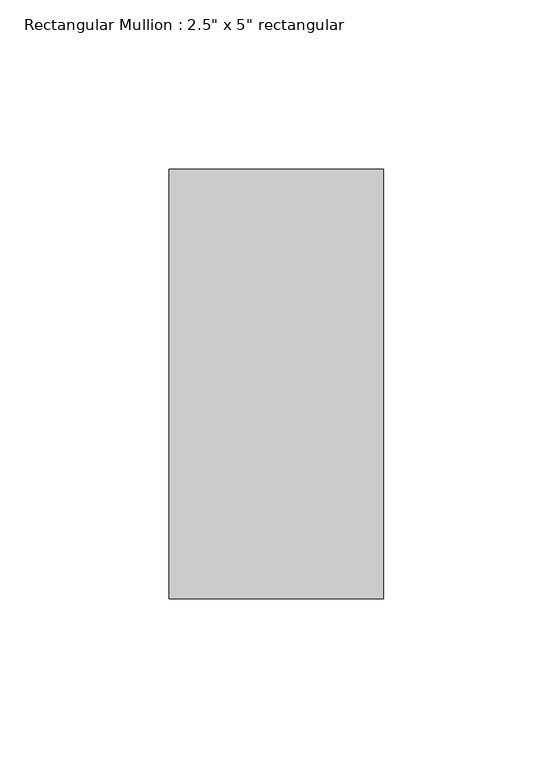
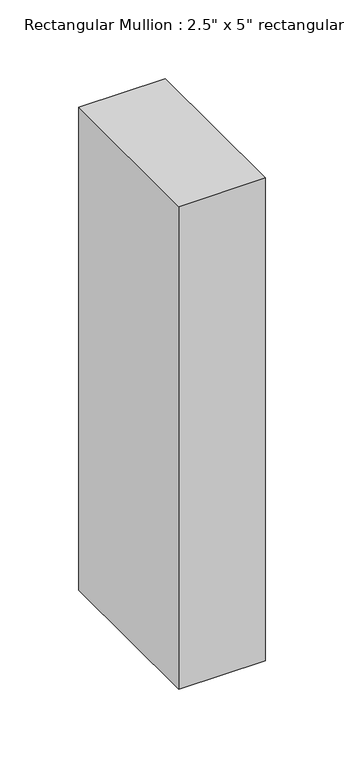
"""IFC4 building model written with IfcOpenShell, lengths in millimetres: member geometry."""

from ifc_helpers import new_model, si_unit, frame, origin, place, context, project, spatial, polyline, outline, extrude, source, transform, mapped, element, save


def member_8d9b4452(model_context):
    return source(origin(), model_context, "Body", "SweptSolid", [
        extrude(outline(polyline([(0.0, 63.5), (0.0, -63.5), (-63.5, -63.5), (-63.5, 63.5), (0.0, 63.5)])), frame((0.0, 0.0, -374.65), z_axis=(0.0, 0.0, 1.0), x_axis=(1.0, 0.0, 0.0)), (0.0, 0.0, 1.0), 374.65),
    ])


if __name__ == "__main__":
    model = new_model("IFC4")
    model_context = context("Model", 3, world=origin())
    ifc_project = project(units=[si_unit("LENGTHUNIT", "METRE", prefix="MILLI")], contexts=[model_context])
    site = spatial("IfcSite", under=ifc_project)
    building = spatial("IfcBuilding", under=site)
    placement = place(None, origin())
    member_shape = member_8d9b4452(model_context)
    element("IfcMember", 1, ObjectType="Rectangular Mullion : 2.5\" x 5\" rectangular", at=placement, inside=building, context=model_context, shape_type="MappedRepresentation", body=[
        mapped(member_shape, transform((0.0, 0.0, 0.0), x_axis=(1.0, 0.0, 0.0), y_axis=(0.0, 1.0, 0.0), z_axis=(0.0, 0.0, 1.0))),
    ])
    save(model, "model.ifc")

# Revit data of these elements
# Type "Rectangular Mullion : 2.5\" x 5\" rectangular"
#   built-in parameter 1007304 = 0.416667 (stored number, unit not read)
#   built-in parameter 1007301 = 0.104167 (stored number, unit not read)
#   built-in parameter 1007300 = 0.104167 (stored number, unit not read)
# Element 1 (IfcMember, "Rectangular Mullion : 2.5\" x 5\" rectangular")
#   Materials on its faces: "Aluminum"
# Materials
#   "Aluminum": class "Metal", colour RGB 247 247 247, transparency 0, Description = "Aluminum 6061", Cost = 0
